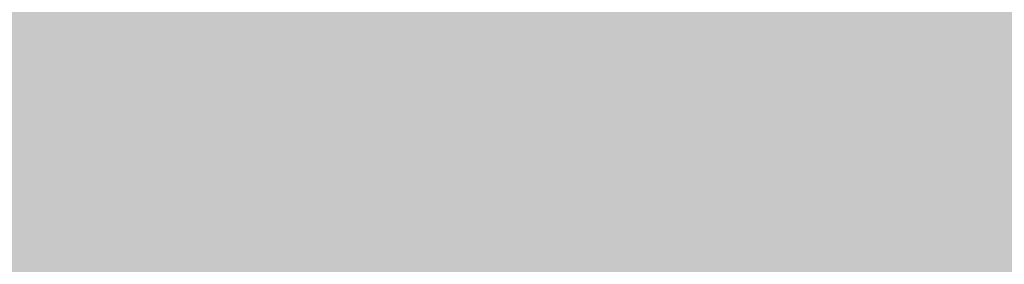
# Model space of a CAD drawing. Units: inches. Extents: x 2083 to 3317, y 1141 to 2115.
# Tile 155 of 256: x 3126.946713 to 3126.955939, y 1263.263648 to 1263.265937. Entities that reach past the tile are written whole.
import ezdxf

# ---------------------------------------------------------------- set-up
doc = ezdxf.new("R2010")
doc.units = ezdxf.units.IN
doc.layers.add('A-ANNO-DIMS', color=2, linetype='Continuous', lineweight=18)
doc.layers.add('A-WALL-PATT', color=251, linetype='Continuous', lineweight=13, true_color=0x636466)
doc.styles.get("Standard").update_dxf_attribs({"font": 'arial.ttf'})
doc.dimstyles.new('ISO-25', dxfattribs={"dimtxt": 12, "dimasz": 12, "dimexe": 1.25, "dimexo": 0.625, "dimtad": 1, "dimlunit": 3, "dimtxsty": 'Standard', "dimcen": 2.5, "dimadec": 0, "dimazin": 0, "dimtfac": 1, "dimtmove": 0, "dimatfit": 3, "dimfxl": 1, "dimarcsym": 0})

# ---------------------------------------------------------------- blocks, each defined once
blk = doc.blocks.new('*D26')
at = {"layer": 'A-ANNO-DIMS', "color": 0, "lineweight": -2, "transparency": 16777216}
for p, q in [((3088.985844, 1274.915092), (3088.985844, 1270.9519631)), ((3111.2400366, 1274.915092), (3111.2400366, 1270.9519631)), ((3076.985844, 1272.2019631), (2840.262447, 1272.2019631)), ((3111.2400366, 1272.2019631), (3088.985844, 1272.2019631)), ((3123.2400366, 1272.2019631), (3135.2400366, 1272.2019631))]:
    blk.add_line(p, q, dxfattribs=at)
at = {"layer": 'A-ANNO-DIMS', "color": 0, "transparency": 16777216}
for points in [[(3076.985844, 1274.2019631), (3076.985844, 1270.2019631), (3088.985844, 1272.2019631)], [(3123.2400366, 1274.2019631), (3123.2400366, 1270.2019631), (3111.2400366, 1272.2019631)]]:
    blk.add_solid(points, dxfattribs=at)
at = {"layer": 'Defpoints', "color": 0, "transparency": 16777216}
for p in [(3088.985844, 1275.540092), (3111.2400366, 1275.540092), (3088.985844, 1272.2019631)]:
    blk.add_point(p, dxfattribs=at)
at = {"layer": 'A-ANNO-DIMS', "color": 0, "transparency": 16777216, "insert": (2952.6241455, 1279.0316016), "char_height": 12, "attachment_point": 5}
blk.add_mtext('NIGHTSTAND 1\'-10 1/2" TYP.', dxfattribs=at)

msp = doc.modelspace()

# ---------------------------------------------------------------- hatches: boundary and pattern name
at = {"layer": 'A-WALL-PATT'}
h = msp.add_hatch(color=256, dxfattribs=at)
h.dxf.hatch_style = 1
h.paths.add_polyline_path([(3126.9597832, 2020.7613601), (2748.9597832, 2020.7613601), (2604.9597832, 2020.7613601), (2226.9597832, 2020.7613601), (2226.9597832, 1702.7613601), (2466.9597832, 1702.7613601), (2466.9597832, 1582.7613601), (2418.9597832, 1582.7613601), (2418.9597832, 1477.7613601), (2226.9597832, 1477.7613601), (2226.9597832, 1263.2613601), (2544.9597832, 1263.2613601), (2544.9597832, 1411.7613601), (2604.9597832, 1411.7613601), (2685.9597832, 1411.7613601), (2685.9597832, 1420.7613601), (2604.9597832, 1420.7613601), (2604.9597832, 1573.7613601), (2604.9597832, 1702.7613601), (2604.9597832, 2011.7613601), (2748.9597832, 2011.7613601), (2748.9597832, 1702.7613601), (2862.9597832, 1702.7613601), (2862.9597832, 1621.7613601), (2871.9597832, 1621.7613601), (2871.9597832, 1702.7613601), (2883.9597832, 1702.7613601), (2883.9597832, 1706.9394595, -0.026459), (2883.9597832, 1711.7613601), (2757.9597832, 1711.7613601), (2757.9597832, 1807.7613601), (2787.9597832, 1807.7613601), (2787.9597832, 1812.2613601), (2757.9597832, 1812.2613601), (2757.9597832, 2011.7613601), (2877.9597832, 2011.7613601), (2877.9597832, 1812.2613601), (2847.9597832, 1812.2613601), (2847.9597832, 1807.7613601), (2889.8357425, 1807.7613601), (2889.8357425, 1812.2613601), (2882.4597832, 1812.2613601), (2882.4597832, 2011.7613601), (3117.9597832, 2011.7613601), (3117.9597832, 1812.2613601), (2937.8357425, 1812.2613601), (2937.8357425, 1807.7613601), (2995.7097832, 1807.7613601), (2995.7097832, 1796.1176655), (3000.2097832, 1796.1176655), (3000.2097832, 1807.7613601), (3117.9597832, 1807.7613601), (3117.9597832, 1711.7613601), (3000.2097832, 1711.7613601), (3000.2097832, 1760.1176655), (2998.5727047, 1760.1176655, -0.020711), (2995.7097832, 1760.1176655), (2995.7097832, 1711.7613601), (2931.9597832, 1711.7613601), (2931.9597832, 1702.7613601), (3126.9597832, 1702.7613601)])
h.paths.add_polyline_path([(2471.4597832, 2011.7613601), (2471.4597832, 1810.0113601), (2462.7169357, 1810.0113601), (2462.7169357, 1805.5113601), (2505.9597832, 1805.5113601), (2505.9597832, 1810.0113601), (2475.9597832, 1810.0113601), (2475.9597832, 2011.7613601), (2595.9597832, 2011.7613601), (2595.9597832, 1810.0113601), (2565.9597832, 1810.0113601), (2565.9597832, 1805.5113601), (2595.9597832, 1805.5113601), (2595.9597832, 1711.7613601), (2235.9597832, 1711.7613601), (2235.9597832, 1805.5113601), (2353.7097832, 1805.5113601), (2353.7097832, 1796.0541624), (2358.2097832, 1796.0541624), (2358.2097832, 1805.5113601), (2414.7169357, 1805.5113601), (2414.7169357, 1810.0113601), (2235.9597832, 1810.0113601), (2235.9597832, 2011.7613601)], flags=16)
h.paths.add_polyline_path([(2270.2047343, 1994.6100082), (2270.2047343, 1970.6100082), (2246.2047343, 1970.6100082), (2246.2047343, 1994.6100082)], flags=0)
edge = h.paths.add_edge_path(flags=0)
edge.add_ellipse((2332.027391, 1899.7981761), major_axis=(-3.0429938, 3.0429938), ratio=0.16825245, start_angle=-161.3321656, end_angle=-156.3071136, ccw=False)
edge.add_ellipse((2333.0820373, 1898.7435297), major_axis=(-1.0546463, 1.0546463), ratio=0.453532097, start_angle=-123.371019, end_angle=-94.1591066)
edge = h.paths.add_edge_path(flags=0)
edge.add_ellipse((2332.027391, 1968.8762897), major_axis=(3.0429938, 3.0429938), ratio=0.16825245, start_angle=18.6678344, end_angle=23.6928864)
edge.add_spline(control_points=[(2332.9255964, 1970.6911045), (2332.2267681, 1970.3360997), (2330.8937087, 1969.6589054), (2328.4130803, 1970.9321376), (2327.2039345, 1967.7487119), (2324.7095965, 1969.9555886), (2322.5328223, 1967.012354), (2320.0128462, 1971.2958124), (2317.6803077, 1968.1578449), (2316.0405263, 1967.1020468), (2315.4269045, 1966.8096022)], knot_values=[0, 0, 0, 0, 2.267059, 4.324559, 6.685584, 8.878641, 11.121502, 14.300359, 17.755284, 19.732645, 19.732645, 19.732645, 19.732645], degree=3, periodic=0)
edge.add_ellipse((2332.027391, 1968.8762897), major_axis=(3.0429938, 3.0429938), ratio=0.16825245, start_angle=18.6678344, end_angle=23.6928864, ccw=False)
edge.add_ellipse((2333.0820373, 1969.930936), major_axis=(1.0546463, 1.0546463), ratio=0.453532097, start_angle=56.628981, end_angle=85.8408934, ccw=False)
edge = h.paths.add_edge_path(flags=0)
edge.add_spline(control_points=[(2296.4282874, 1967.9879081), (2293.6278045, 1965.3363137), (2287.7036238, 1959.727094), (2299.7438601, 1949.9956993), (2294.5325909, 1935.6685275), (2290.5732281, 1920.6035119), (2293.3941244, 1909.9736911), (2296.1854073, 1904.9665431)], knot_values=[0.099185, 0.099185, 0.099185, 0.099185, 0.345301, 0.619822, 0.982653, 1.386093, 1.810555, 1.810555, 1.810555, 1.810555], degree=3, periodic=0)
edge.add_spline(control_points=[(2296.1854073, 1904.9665431), (2297.3835817, 1902.6193002), (2298.0009694, 1901.9493116), (2298.5529698, 1901.4681549)], knot_values=[0.006246, 0.006246, 0.006246, 0.006246, 0.055476, 0.055476, 0.055476, 0.055476], degree=3, periodic=0)
edge.add_spline(control_points=[(2298.5529698, 1901.4681549), (2297.2586121, 1900.9232238), (2295.2252939, 1900.2321257), (2293.0602287, 1900.6142053), (2292.1014227, 1900.788415), (2292.0895776, 1900.790568)], knot_values=[0.312835, 0.312835, 0.312835, 0.312835, 0.40178, 0.474987, 0.475903, 0.475903, 0.475903, 0.475903], degree=3, periodic=0)
edge.add_arc((2292.7936464, 1904.6641088), 3.9370079, 215.4208969, 259.6981795, ccw=False)
edge.add_spline(control_points=[(2289.5853139, 1902.3823039), (2289.4766524, 1902.5350874), (2289.3684805, 1902.6880353), (2289.2608648, 1902.8411699)], knot_values=[0.102872, 0.102872, 0.102872, 0.102872, 0.116896, 0.116896, 0.116896, 0.116896], degree=3, periodic=0)
edge.add_spline(control_points=[(2289.2608648, 1902.8411699), (2288.6866042, 1902.5501922), (2287.6400477, 1902.0199025), (2285.8813368, 1901.8739536), (2283.8529717, 1901.5043521), (2281.7199871, 1899.7105375), (2278.4669913, 1899.492942), (2276.1571361, 1901.8832022), (2272.2589526, 1899.8040711), (2267.7776054, 1901.8431828), (2262.2438819, 1900.1840326), (2257.414927, 1901.7820606), (2254.318374, 1900.7261196), (2253.1782849, 1900.3373431)], knot_values=[0, 0, 0, 0, 1.907977, 3.477176, 5.261074, 7.972851, 11.680248, 13.717921, 16.939592, 22.789562, 27.502503, 33.595215, 37.145618, 37.145618, 37.145618, 37.145618], degree=3, periodic=0)
edge.add_line((2253.1782849, 1900.3373431), (2250.2442397, 1902.8411699))
edge.add_line((2250.2442397, 1902.8411699), (2250.2442397, 1965.8332959))
edge.add_line((2250.2442397, 1965.8332959), (2253.1782849, 1968.3371226))
edge.add_spline(control_points=[(2253.1782849, 1968.3371226), (2254.318374, 1967.9483462), (2257.414927, 1966.8924051), (2262.2438819, 1968.4904332), (2267.7776054, 1966.8312829), (2271.5267301, 1968.5372172), (2273.8759143, 1967.8282895), (2274.2067012, 1967.7276424)], knot_values=[0, 0, 0, 0, 0.09018, 0.244935, 0.364644, 0.513233, 0.537855, 0.537855, 0.537855, 0.537855], degree=3, periodic=0)
edge.add_arc((2274.3528869, 1963.7933495), 3.9370079, 72.0511336, 92.1279492, ccw=False)
edge.add_arc((2281.2969331, 1985.2300027), 18.5962982, 252.05113361, 288.56572166)
edge.add_arc((2292.3167172, 1956.0288805), 12.6460805, 71.02678788, 113.77821843, ccw=False)
edge = h.paths.add_edge_path(flags=0)
edge.add_spline(control_points=[(2274.8994147, 1951.8561946), (2275.066156, 1951.6165924), (2275.2326866, 1951.3765878), (2275.3979871, 1951.1358545)], knot_values=[1.409916, 1.409916, 1.409916, 1.409916, 1.43159, 1.43159, 1.43159, 1.43159], degree=3, periodic=0)
edge.add_spline(control_points=[(2275.3979871, 1951.1358545), (2275.7921055, 1950.5618854), (2276.1792311, 1949.9837745), (2276.5455462, 1949.3971029)], knot_values=[1.358238, 1.358238, 1.358238, 1.358238, 1.409916, 1.409916, 1.409916, 1.409916], degree=3, periodic=0)
edge.add_line((2276.5455462, 1949.3971029), (2277.437289, 1947.8621847))
edge.add_spline(control_points=[(2277.437289, 1947.8621847), (2276.3038341, 1945.6731147), (2274.6396979, 1942.4268817), (2274.631615, 1938.0938998), (2272.7991237, 1930.8515498), (2274.3564261, 1943.8970461), (2275.9476814, 1947.9233558), (2276.5455462, 1949.3971029)], knot_values=[0.005632, 0.005632, 0.005632, 0.005632, 0.186014, 0.266002, 0.357087, 0.59639, 0.739732, 0.739732, 0.739732, 0.739732], degree=3, periodic=0)
edge.add_spline(control_points=[(2276.5455462, 1949.3971029), (2276.1792311, 1949.9837745), (2275.7921055, 1950.5618854), (2275.3979871, 1951.1358545)], knot_values=[1.358238, 1.358238, 1.358238, 1.358238, 1.409916, 1.409916, 1.409916, 1.409916], degree=3, periodic=0)
edge.add_spline(control_points=[(2275.3979871, 1951.1358545), (2274.9425002, 1950.0804523), (2274.2077604, 1948.0252718), (2273.9346018, 1944.8514774), (2272.4685341, 1937.6274891), (2273.4662155, 1945.6964663), (2274.7006154, 1951.0594725), (2274.8994147, 1951.8561946)], knot_values=[0.104364, 0.104364, 0.104364, 0.104364, 0.189636, 0.269624, 0.36071, 0.600013, 0.644622, 0.644622, 0.644622, 0.644622], degree=3, periodic=0)
h.paths.add_polyline_path([(2269.1675139, 1963.1275729, -0.357527), (2268.170633, 1960.9763695, -0.092561), (2268.170633, 1939.4363249, -0.357527), (2269.1675139, 1937.2851215, -0.357527), (2267.0163105, 1938.2820024, -0.164785), (2254.6855813, 1938.2820024, -0.357527), (2252.5343779, 1937.2851215, -0.357527), (2253.5312587, 1939.4363249, -0.092561), (2253.5312587, 1960.9763695, -0.357527), (2252.5343779, 1963.1275729, -0.357527), (2254.6855813, 1962.130692, -0.164785), (2267.0163105, 1962.130692, -0.357527)], flags=0)
h.paths.add_polyline_path([(2248.8740679, 1967.8017998), (2248.8740679, 1957.0277095), (2249.4577833, 1957.0277095), (2249.4577833, 1911.6467562), (2248.8740679, 1911.6467562), (2248.8740679, 1900.8726659), (2246.5118632, 1900.8726659, 0.197327), (2244.1496584, 1902.4568734), (2244.1496584, 1966.2175923, 0.197327), (2246.5118632, 1967.8017998)], flags=0)
h.paths.add_polyline_path([(2269.1675139, 1931.3893442, -0.357527), (2268.170633, 1929.2381408, -0.092561), (2268.170633, 1907.6980962, -0.357527), (2269.1675139, 1905.5468928, -0.357527), (2267.0163105, 1906.5437737, -0.164785), (2254.6855813, 1906.5437737, -0.357527), (2252.5343779, 1905.5468928, -0.357527), (2253.5312587, 1907.6980962, -0.092561), (2253.5312587, 1929.2381408, -0.357527), (2252.5343779, 1931.3893442, -0.357527), (2254.6855813, 1930.3924634, -0.164785), (2267.0163105, 1930.3924634, -0.357527)], flags=0)
edge = h.paths.add_edge_path(flags=0)
edge.add_spline(control_points=[(2276.1968578, 1906.7237016), (2276.1681442, 1909.0289278), (2276.1140492, 1913.371852), (2270.5984171, 1924.9249783), (2273.9051746, 1919.0127787), (2275.9217115, 1916.2620626), (2275.4745699, 1912.4021495), (2277.2578735, 1910.3806206), (2276.6960436, 1908.2250358), (2276.6462176, 1906.8130226), (2276.6178249, 1906.0084068)], knot_values=[0, 0, 0, 0, 8.61026, 16.221274, 18.843057, 23.804898, 27.440828, 29.356102, 31.203478, 33.650687, 33.650687, 33.650687, 33.650687], degree=3, periodic=0)
edge.add_spline(control_points=[(2276.6178249, 1906.0084068), (2276.6233131, 1905.6241436), (2276.4977381, 1904.6286608), (2275.4417789, 1903.8547251), (2274.9373144, 1903.0804497), (2274.8590804, 1902.8411699)], knot_values=[0.156488, 0.156488, 0.156488, 0.156488, 0.184398, 0.231376, 0.250598, 0.250598, 0.250598, 0.250598], degree=3, periodic=0)
edge.add_line((2274.8590804, 1902.8411699), (2276.50598, 1902.8411699))
edge.add_spline(control_points=[(2276.50598, 1902.8411699), (2276.7883084, 1903.0849395), (2277.6650711, 1904.1251958), (2278.2495378, 1904.340738), (2277.6538719, 1908.5273866), (2278.15567, 1906.2278078), (2278.100464, 1905.2859484), (2278.8466748, 1904.0690054), (2277.8567853, 1903.4149482), (2277.8741909, 1902.9910497), (2277.9035616, 1902.8411699)], knot_values=[0.059574, 0.059574, 0.059574, 0.059574, 0.080753, 0.103741, 0.16972, 0.176036, 0.207137, 0.240474, 0.262341, 0.27366, 0.27366, 0.27366, 0.27366], degree=3, periodic=0)
edge.add_line((2277.9035616, 1902.8411699), (2280.0298255, 1902.8411699))
edge.add_spline(control_points=[(2280.0298255, 1902.8411699), (2279.8882214, 1903.088398), (2279.4992571, 1903.9815512), (2280.1522839, 1905.9393491), (2278.103615, 1909.6577572), (2279.7623946, 1907.185285), (2280.3279002, 1904.8748608), (2280.4851086, 1903.4895904), (2281.4632687, 1903.2494323), (2281.7583431, 1902.9364967), (2281.8340361, 1902.8411699)], knot_values=[0.013856, 0.013856, 0.013856, 0.013856, 0.034874, 0.088867, 0.107879, 0.126738, 0.158714, 0.193757, 0.217487, 0.226722, 0.226722, 0.226722, 0.226722], degree=3, periodic=0)
edge.add_spline(control_points=[(2281.8340361, 1902.8411699), (2281.7875348, 1902.8267029), (2281.6470224, 1902.7829881), (2281.3955272, 1902.85949), (2281.088077, 1902.9852418), (2280.7206826, 1903.060902), (2280.3334513, 1903.0257257), (2280.1247668, 1902.898879), (2280.0298255, 1902.8411699)], knot_values=[0, 0, 0, 0, 0.14413, 0.435517, 0.749276, 1.153046, 1.548371, 1.878348, 1.878348, 1.878348, 1.878348], degree=3, periodic=0)
edge.add_line((2280.0298255, 1902.8411699), (2277.9035616, 1902.8411699))
edge.add_spline(control_points=[(2277.9035616, 1902.8411699), (2277.892855, 1902.7958553), (2277.865396, 1902.6796374), (2277.6074793, 1902.6874828), (2277.2740503, 1902.8006999), (2276.8379209, 1902.6197745), (2276.5838074, 1902.7892611), (2276.50598, 1902.8411699)], knot_values=[0, 0, 0, 0, 0.127189, 0.326199, 0.628009, 1.24357, 1.515331, 1.515331, 1.515331, 1.515331], degree=3, periodic=0)
edge.add_line((2276.50598, 1902.8411699), (2274.8590804, 1902.8411699))
edge.add_spline(control_points=[(2274.8590804, 1902.8411699), (2274.8144367, 1902.8985868), (2274.7251297, 1903.013446), (2274.4934765, 1903.1189684), (2274.2442854, 1902.9605386), (2273.9371207, 1903.1849416), (2273.6140395, 1902.9831428), (2273.4083164, 1902.8830449), (2273.322254, 1902.8411699)], knot_values=[0, 0, 0, 0, 0.21843, 0.436957, 0.687977, 0.990379, 1.398396, 1.69185, 1.69185, 1.69185, 1.69185], degree=3, periodic=0)
edge.add_spline(control_points=[(2273.322254, 1902.8411699), (2273.6167403, 1903.445692), (2274.2739977, 1904.5382529), (2276.0272387, 1904.5737017), (2276.2069634, 1906.5836372), (2276.1968578, 1906.7237016)], knot_values=[0.012227, 0.012227, 0.012227, 0.012227, 0.059472, 0.106218, 0.134458, 0.134458, 0.134458, 0.134458], degree=3, periodic=0)
h.paths.add_polyline_path([(2270.7760538, 1897.7898284), (2270.7760538, 1873.7898284), (2246.7760538, 1873.7898284), (2246.7760538, 1897.7898284)], flags=0)
h.paths.add_polyline_path([(2353.7097832, 1760.0050593), (2353.7097832, 1760.0541624), (2358.2097832, 1760.0541624, -0.033729)], flags=0)
h.paths.add_polyline_path([(2321.8191188, 1737.5291862), (2341.9953271, 1737.5291862, -0.414214), (2343.2032727, 1736.3212406), (2343.2032727, 1721.0205964, -0.414214), (2341.9953271, 1719.8126508), (2321.8191188, 1719.8126508, -0.414214), (2320.6111732, 1721.0205964), (2320.6111732, 1736.3212406, -0.414214)], flags=0)
h.paths.add_polyline_path([(2324.2350099, 1736.3212406), (2339.5794359, 1736.3212406, -0.414214), (2341.9953271, 1733.9053494), (2341.9953271, 1725.4497302, -0.414214), (2339.5794359, 1723.033839), (2333.6805885, 1723.033839), (2333.8453172, 1722.0454666, -0.870646), (2335.4253988, 1721.8258934, -0.767327), (2333.922694, 1721.4232449), (2331.2910241, 1721.4232449, -0.767327), (2329.7883193, 1721.8258934, -0.870646), (2331.3684009, 1722.0454666), (2331.5331296, 1723.033839), (2324.2350099, 1723.033839, -0.414214), (2321.8191188, 1725.4497302), (2321.8191188, 1733.9053494, -0.414214)], flags=0)
h.paths.add_polyline_path([(2570.4837892, 1928.6154443), (2589.6837892, 1928.6154443), (2590.1688286, 1928.6154443), (2590.1688286, 1904.9933971), (2570.4837892, 1904.9933971)], flags=0)
h.paths.add_polyline_path([(2574.4473242, 1927.2638215, -1), (2572.8288357, 1927.2638215, -1)], flags=0)
h.paths.add_polyline_path([(2573.0898665, 1926.9408768), (2573.925032, 1927.7760423), (2574.1477428, 1927.5533315), (2573.3125773, 1926.718166)], flags=0)
h.paths.add_polyline_path([(2578.7790648, 1919.7296175, -1), (2571.5916632, 1919.7296175, -1)], flags=0)
h.paths.add_polyline_path([(2578.385364, 1919.7296175, -1), (2571.985364, 1919.7296175, -1)], flags=0)
h.paths.add_polyline_path([(2331.5957638, 1729.4762156, -1), (2333.6179542, 1729.4762156, -1)], flags=0)
h.paths.add_polyline_path([(2578.0342282, 1927.2638215, -1), (2576.4157396, 1927.2638215, -1)], flags=0)
h.paths.add_polyline_path([(2576.6888513, 1927.5310886), (2576.9115621, 1927.7537993), (2577.7467276, 1926.9186339), (2577.5240168, 1926.6959231)], flags=0)
h.paths.add_polyline_path([(2578.1390648, 1909.8595388, -1), (2572.2316632, 1909.8595388, -1)], flags=0)
h.paths.add_polyline_path([(2577.745364, 1909.8595388, -1), (2572.625364, 1909.8595388, -1)], flags=0)
h.paths.add_polyline_path([(2583.7977179, 1927.2638215, -1), (2582.1792294, 1927.2638215, -1)], flags=0)
h.paths.add_polyline_path([(2582.7186487, 1927.7537993), (2583.5538142, 1926.9186339), (2583.3311034, 1926.6959231), (2582.4959379, 1927.5310886)], flags=0)
h.paths.add_polyline_path([(2582.4959379, 1927.5310886), (2582.7186487, 1927.7537993), (2583.5538142, 1926.9186339), (2583.3311034, 1926.6959231)], flags=0)
h.paths.add_polyline_path([(2587.7390648, 1920.5296175, -1), (2581.8316632, 1920.5296175, -1)], flags=0)
h.paths.add_polyline_path([(2587.345364, 1920.5296175, -1), (2582.225364, 1920.5296175, -1)], flags=0)
h.paths.add_polyline_path([(2587.3846219, 1927.2638215, -1), (2585.7661333, 1927.2638215, -1)], flags=0)
h.paths.add_polyline_path([(2586.0819925, 1926.9802469), (2586.917158, 1927.8154124), (2587.1398688, 1927.5927016), (2586.3047033, 1926.7575361)], flags=0)
h.paths.add_polyline_path([(2588.3790648, 1910.6595388, -1), (2581.1916632, 1910.6595388, -1)], flags=0)
h.paths.add_polyline_path([(2587.985364, 1910.6595388, -1), (2581.585364, 1910.6595388, -1)], flags=0)
h.paths.add_polyline_path([(2417.1677288, 1729.4778955), (2437.3439372, 1729.4778955, -0.414214), (2438.5518828, 1728.2699499), (2438.5518828, 1712.9693057, -0.414214), (2437.3439372, 1711.7613601), (2417.1677288, 1711.7613601, -0.414214), (2415.9597832, 1712.9693057), (2415.9597832, 1728.2699499, -0.414214)], flags=0)
h.paths.add_polyline_path([(2419.58362, 1728.2699499), (2434.928046, 1728.2699499, -0.414214), (2437.3439372, 1725.8540587), (2437.3439372, 1717.3984395, -0.414214), (2434.928046, 1714.9825483), (2429.0291985, 1714.9825483), (2429.1939273, 1713.9941758, -0.870646), (2430.7740089, 1713.7746027, -0.767327), (2429.2713041, 1713.3719542), (2426.6396342, 1713.3719542, -0.767327), (2425.1369294, 1713.7746027, -0.870646), (2426.717011, 1713.9941758), (2426.8817397, 1714.9825483), (2419.58362, 1714.9825483, -0.414214), (2417.1677288, 1717.3984395), (2417.1677288, 1725.8540587, -0.414214)], flags=0)
h.paths.add_polyline_path([(2419.58362, 1728.2699499), (2434.928046, 1728.2699499, -0.414214), (2437.3439372, 1725.8540587), (2437.3439372, 1717.3984395, -0.414214), (2434.928046, 1714.9825483), (2429.0291985, 1714.9825483), (2428.3581177, 1719.0090337), (2427.5528206, 1719.0090337), (2426.8817397, 1714.9825483), (2419.58362, 1714.9825483, -0.414214), (2417.1677288, 1717.3984395), (2417.1677288, 1725.8540587, -0.414214)], flags=0)
h.paths.add_polyline_path([(2426.9443739, 1721.4249248, -1), (2428.9665643, 1721.4249248, -1)], flags=0)
h.paths.add_polyline_path([(2475.9597832, 1702.7613601), (2595.9597832, 1702.7613601), (2595.9597832, 1582.7613601), (2475.9597832, 1582.7613601)], flags=16)
h.paths.add_polyline_path([(2427.9597832, 1573.7613601), (2595.9597832, 1573.7613601), (2595.9597832, 1468.7613601), (2595.9597832, 1420.7613601), (2384.4597832, 1420.7613601), (2384.4597832, 1468.7613601), (2427.9597832, 1468.7613601)], flags=16)
h.paths.add_polyline_path([(2379.9597832, 1468.7613601), (2379.9597832, 1420.7613601), (2235.9597832, 1420.7613601), (2235.9597832, 1468.7613601)], flags=16)
h.paths.add_polyline_path([(2317.8159962, 1466.695767), (2337.9922045, 1466.695767, -0.414214), (2339.2001501, 1465.4878214), (2339.2001501, 1450.1871771, -0.414214), (2337.9922045, 1448.9792315), (2317.8159962, 1448.9792315, -0.414214), (2316.6080506, 1450.1871771), (2316.6080506, 1465.4878214, -0.414214)], flags=0)
h.paths.add_polyline_path([(2320.2318874, 1465.4878214), (2335.5763133, 1465.4878214, -0.414214), (2337.9922045, 1463.0719302), (2337.9922045, 1454.616311, -0.414214), (2335.5763133, 1452.2004198), (2329.6774659, 1452.2004198), (2329.8421946, 1451.2120473, -0.870646), (2331.4222762, 1450.9924742, -0.767327), (2329.9195714, 1450.5898257), (2327.2879015, 1450.5898257, -0.767327), (2325.7851967, 1450.9924742, -0.870646), (2327.3652783, 1451.2120473), (2327.530007, 1452.2004198), (2320.2318874, 1452.2004198, -0.414214), (2317.8159962, 1454.616311), (2317.8159962, 1463.0719302, -0.414214)], flags=0)
h.paths.add_polyline_path([(2320.2318874, 1465.4878214), (2335.5763133, 1465.4878214, -0.414214), (2337.9922045, 1463.0719302), (2337.9922045, 1454.616311, -0.414214), (2335.5763133, 1452.2004198), (2329.6774659, 1452.2004198), (2329.006385, 1456.2269051), (2328.2010879, 1456.2269051), (2327.530007, 1452.2004198), (2320.2318874, 1452.2004198, -0.414214), (2317.8159962, 1454.616311), (2317.8159962, 1463.0719302, -0.414214)], flags=0)
h.paths.add_polyline_path([(2327.5926413, 1458.6427963, -1), (2329.6148317, 1458.6427963, -1)], flags=0)
h.paths.add_polyline_path([(2244.4117436, 1433.3404531), (2241.9209449, 1433.3404531, -0.414214), (2240.0178562, 1435.2435418), (2240.0178562, 1440.9528078, -0.414211), (2241.920925, 1442.8558965), (2244.4117436, 1442.8558965, -1.976472)], flags=0)
h.paths.add_polyline_path([(2245.3568884, 1434.3975358, -0.414214), (2245.3568884, 1441.7988138, -2.144098)], flags=0)
h.paths.add_polyline_path([(2535.9597832, 1416.2613601), (2535.9597832, 1272.2613601), (2235.9597832, 1272.2613601), (2235.9597832, 1416.2613601)], flags=16)
h.paths.add_polyline_path([(2260.1195614, 1384.2928413), (2260.1195614, 1362.0386487), (2237.8653688, 1362.0386487), (2237.8653688, 1384.2928413)], flags=0)
edge = h.paths.add_edge_path(flags=0)
edge.add_line((2318.2518466, 1362.0932983), (2318.1457968, 1362.0009726))
edge.add_ellipse((2317.4451158, 1360.4310442), major_axis=(2.8216404, 2.8216404), ratio=0.16825245, start_angle=18.6678344, end_angle=20.9481273, ccw=False)
edge.add_ellipse((2318.4230451, 1361.4089735), major_axis=(0.9779293, 0.9779293), ratio=0.453532097, start_angle=56.628981, end_angle=70.2262012, ccw=False)
edge = h.paths.add_edge_path(flags=0)
edge.add_line((2319.1073699, 1295.5710784), (2319.0150442, 1295.6771282))
edge.add_ellipse((2317.4451158, 1296.3778091), major_axis=(-2.8216404, 2.8216404), ratio=0.16825245, start_angle=-161.3321656, end_angle=-159.0518727, ccw=False)
edge.add_ellipse((2318.4230451, 1295.3998798), major_axis=(-0.9779293, 0.9779293), ratio=0.453532097, start_angle=-123.371019, end_angle=-109.7737988)
edge = h.paths.add_edge_path(flags=0)
edge.add_spline(control_points=[(2284.2103489, 1301.1702189), (2284.5806878, 1300.444719), (2284.8911891, 1299.8920243), (2285.159553, 1299.4610182)], knot_values=[0.039066, 0.039066, 0.039066, 0.039066, 0.055476, 0.055476, 0.055476, 0.055476], degree=3, periodic=0)
edge.add_line((2285.159553, 1299.4610182), (2284.2103489, 1301.1702189))
edge = h.paths.add_edge_path(flags=0)
edge.add_line((2280.4124579, 1297.2980125), (2283.3699905, 1297.0361216))
edge.add_line((2283.3699905, 1297.0361216), (2286.4056902, 1297.9263104))
edge.add_spline(control_points=[(2286.4056902, 1297.9263104), (2285.305487, 1297.4631193), (2284.3447774, 1297.1291508), (2283.3699905, 1297.0361216)], knot_values=[0.394369, 0.394369, 0.394369, 0.394369, 0.475903, 0.475903, 0.475903, 0.475903], degree=3, periodic=0)
edge.add_spline(control_points=[(2283.3699905, 1297.0361216), (2283.2813895, 1297.027666), (2282.316289, 1296.9573356), (2281.3125019, 1297.1344787), (2280.4234414, 1297.2960161), (2280.4124579, 1297.2980125)], knot_values=[0.312835, 0.312835, 0.312835, 0.312835, 0.320246, 0.393453, 0.394369, 0.394369, 0.394369, 0.394369], degree=3, periodic=0)
edge = h.paths.add_edge_path(flags=0)
edge.add_line((2284.4355615, 1359.6072854), (2280.4462909, 1355.328047))
edge.add_line((2280.4462909, 1355.328047), (2279.5799868, 1351.0177544))
edge.add_line((2279.5799868, 1351.0177544), (2282.4129737, 1346.5804327))
edge.add_spline(control_points=[(2282.4129737, 1346.5804327), (2283.1533308, 1345.5892358), (2284.2528957, 1344.0288973), (2284.801037, 1342.3871671), (2284.9351625, 1341.8055443)], knot_values=[1.240098, 1.240098, 1.240098, 1.240098, 1.332892, 1.382712, 1.382712, 1.382712, 1.382712], degree=3, periodic=0)
edge.add_spline(control_points=[(2284.9351625, 1341.8055443), (2285.3191079, 1340.1406002), (2285.2330291, 1338.4092041), (2284.9099384, 1336.6541222)], knot_values=[1.097484, 1.097484, 1.097484, 1.097484, 1.240098, 1.240098, 1.240098, 1.240098], degree=3, periodic=0)
edge.add_spline(control_points=[(2284.9099384, 1336.6541222), (2284.5868478, 1334.8990403), (2284.0267453, 1333.1202725), (2283.4626437, 1331.3605849)], knot_values=[0.95487, 0.95487, 0.95487, 0.95487, 1.097484, 1.097484, 1.097484, 1.097484], degree=3, periodic=0)
edge.add_line((2283.4626437, 1331.3605849), (2281.8903759, 1326.153357))
edge.add_line((2281.8903759, 1326.153357), (2280.7562592, 1321.0560888))
edge.add_line((2280.7562592, 1321.0560888), (2280.2992048, 1316.0019772))
edge.add_line((2280.2992048, 1316.0019772), (2280.7159327, 1310.9500678))
edge.add_line((2280.7159327, 1310.9500678), (2282.0280939, 1305.9721367))
edge.add_line((2282.0280939, 1305.9721367), (2284.2103489, 1301.1702189))
edge.add_spline(control_points=[(2284.2103489, 1301.1702189), (2283.3407305, 1302.7301854), (2282.6119044, 1304.3364933), (2282.0280939, 1305.9721367)], knot_values=[0.099185, 0.099185, 0.099185, 0.099185, 0.241799, 0.241799, 0.241799, 0.241799], degree=3, periodic=0)
edge.add_spline(control_points=[(2282.0280939, 1305.9721367), (2281.4442835, 1307.6077801), (2281.0054886, 1309.2727591), (2280.7159327, 1310.9500678)], knot_values=[0.241799, 0.241799, 0.241799, 0.241799, 0.384413, 0.384413, 0.384413, 0.384413], degree=3, periodic=0)
edge.add_spline(control_points=[(2280.7159327, 1310.9500678), (2280.4332411, 1312.5876134), (2280.2893863, 1314.2769594), (2280.2988938, 1315.9620324), (2280.2992048, 1316.0019772)], knot_values=[0.384413, 0.384413, 0.384413, 0.384413, 0.523647, 0.527028, 0.527028, 0.527028, 0.527028], degree=3, periodic=0)
edge.add_spline(control_points=[(2280.2992048, 1316.0019772), (2280.3123257, 1317.6869552), (2280.4778706, 1319.3679256), (2280.7562592, 1321.0560888)], knot_values=[0.527028, 0.527028, 0.527028, 0.527028, 0.669642, 0.669642, 0.669642, 0.669642], degree=3, periodic=0)
edge.add_spline(control_points=[(2280.7562592, 1321.0560888), (2281.0346478, 1322.7442519), (2281.4258801, 1324.4396079), (2281.8903759, 1326.153357)], knot_values=[0.669642, 0.669642, 0.669642, 0.669642, 0.812256, 0.812256, 0.812256, 0.812256], degree=3, periodic=0)
edge.add_spline(control_points=[(2281.8903759, 1326.153357), (2282.2643834, 1327.5332507), (2282.7878702, 1329.2618097), (2283.352751, 1331.0177803), (2283.4626437, 1331.3605849)], knot_values=[0.812256, 0.812256, 0.812256, 0.812256, 0.927087, 0.95487, 0.95487, 0.95487, 0.95487], degree=3, periodic=0)
edge.add_line((2283.4626437, 1331.3605849), (2284.9099384, 1336.6541222))
edge.add_line((2284.9099384, 1336.6541222), (2284.9351625, 1341.8055443))
edge.add_line((2284.9351625, 1341.8055443), (2282.4129737, 1346.5804327))
edge.add_spline(control_points=[(2282.4129737, 1346.5804327), (2281.2751273, 1348.1037918), (2280.0784467, 1349.5703178), (2279.5799868, 1351.0177544)], knot_values=[1.382712, 1.382712, 1.382712, 1.382712, 1.525326, 1.525326, 1.525326, 1.525326], degree=3, periodic=0)
edge.add_spline(control_points=[(2279.5799868, 1351.0177544), (2279.4432818, 1351.4147209), (2279.1363124, 1352.856922), (2279.7351897, 1354.2903851), (2280.4462909, 1355.328047)], knot_values=[1.525326, 1.525326, 1.525326, 1.525326, 1.564439, 1.667941, 1.667941, 1.667941, 1.667941], degree=3, periodic=0)
edge.add_spline(control_points=[(2280.4462909, 1355.328047), (2281.4261132, 1356.7578354), (2282.9308373, 1358.1825604), (2284.4355615, 1359.6072854)], knot_values=[1.667941, 1.667941, 1.667941, 1.667941, 1.810555, 1.810555, 1.810555, 1.810555], degree=3, periodic=0)
edge.add_arc((2280.6230749, 1348.518181), 11.7261796, 71.02678788, 113.77821843)
edge.add_arc((2270.4048917, 1375.5951559), 17.2435667, 252.05113361, 288.56572166, ccw=False)
edge.add_arc((2263.9659692, 1355.7178471), 3.6506221, 72.0511336, 92.1279492)
edge.add_arc((2263.9659692, 1355.7178471), 3.6506221, 92.1279492, 177.98513)
edge.add_spline(control_points=[(2260.3176041, 1355.8461989), (2260.2604169, 1354.2206683), (2260.551278, 1350.1865469), (2262.9993445, 1346.7662507), (2264.4727415, 1344.6490245)], knot_values=[1.43159, 1.43159, 1.43159, 1.43159, 1.564144, 1.770695, 1.770695, 1.770695, 1.770695], degree=3, periodic=0)
edge.add_line((2264.4727415, 1344.6490245), (2264.9355904, 1343.9825301))
edge.add_spline(control_points=[(2263.8010444, 1340.2481052), (2263.8432379, 1340.5140884), (2264.0672444, 1341.7564652), (2264.5126928, 1343.0024532), (2264.9350468, 1343.9810834)], knot_values=[0.53657, 0.53657, 0.53657, 0.53657, 0.559349, 0.644622, 0.644622, 0.644622, 0.644622], degree=3, periodic=0)
edge.add_spline(control_points=[(2264.9350468, 1343.9810834), (2265.1177715, 1343.7149747), (2265.2988751, 1343.4479058), (2265.4767562, 1343.1793646)], knot_values=[1.384077, 1.384077, 1.384077, 1.384077, 1.409916, 1.409916, 1.409916, 1.409916], degree=3, periodic=0)
edge.add_spline(control_points=[(2265.4767562, 1343.1793646), (2265.6546373, 1342.9108234), (2265.8292958, 1342.64081), (2265.9991301, 1342.368812)], knot_values=[1.358238, 1.358238, 1.358238, 1.358238, 1.384077, 1.384077, 1.384077, 1.384077], degree=3, periodic=0)
edge.add_line((2265.9991301, 1342.368812), (2266.8260057, 1340.9455468))
edge.add_spline(control_points=[(2266.8260057, 1340.9455468), (2268.894401, 1337.0896912), (2271.3981727, 1325.8430009), (2270.5161644, 1310.5685568), (2275.9193759, 1301.860609), (2277.7895113, 1299.1994495)], knot_values=[0.116896, 0.116896, 0.116896, 0.116896, 0.472987, 1.050969, 1.313793, 1.313793, 1.313793, 1.313793], degree=3, periodic=0)
edge.add_spline(control_points=[(2277.7895113, 1299.1994495), (2277.8394051, 1299.1284519), (2277.8894277, 1299.0574975), (2277.9395717, 1298.9865839)], knot_values=[0.109884, 0.109884, 0.109884, 0.109884, 0.116896, 0.116896, 0.116896, 0.116896], degree=3, periodic=0)
edge.add_line((2277.9395717, 1298.9865839), (2277.7888489, 1299.1991139))
edge.add_spline(control_points=[(2277.7888489, 1299.1991139), (2277.2565819, 1298.9294144), (2276.2863504, 1298.4379024), (2275.0393517, 1298.3344186), (2274.3833299, 1298.2388951), (2274.2152543, 1298.209338)], knot_values=[33.12187, 33.12187, 33.12187, 33.12187, 35.029056, 36.598255, 37.144827, 37.144827, 37.144827, 37.144827], degree=3, periodic=0)
edge.add_line((2274.2152543, 1298.209338), (2273.073147, 1297.8929607))
edge.add_spline(control_points=[(2273.073147, 1297.8929607), (2272.3229363, 1297.579784), (2271.0391507, 1296.5105078), (2269.2483948, 1296.2260622), (2268.4231004, 1296.3746543)], knot_values=[26.532584, 26.532584, 26.532584, 26.532584, 29.198919, 31.839101, 31.839101, 31.839101, 31.839101], degree=3, periodic=0)
edge.add_line((2268.4231004, 1296.3746543), (2263.8785014, 1297.4575338))
edge.add_spline(control_points=[(2263.8785014, 1297.4575338), (2263.5560769, 1297.3594345), (2261.8603064, 1296.8386943), (2260.2387805, 1297.2824073), (2258.9334543, 1297.5164611)], knot_values=[15.919551, 15.919551, 15.919551, 15.919551, 16.939592, 21.226067, 21.226067, 21.226067, 21.226067], degree=3, periodic=0)
edge.add_line((2258.9334543, 1297.5164611), (2254.0552332, 1297.3290098))
edge.add_spline(control_points=[(2254.0552332, 1297.3290098), (2253.7555255, 1297.295815), (2252.1136834, 1297.1651738), (2250.4618687, 1297.5442209), (2249.1296862, 1297.6678818)], knot_values=[5.306517, 5.306517, 5.306517, 5.306517, 6.276435, 10.613034, 10.613034, 10.613034, 10.613034], degree=3, periodic=0)
edge.add_line((2249.1296862, 1297.6678818), (2244.3316495, 1296.8777561))
edge.add_line((2244.3316495, 1296.8777561), (2241.6110326, 1299.1994495))
edge.add_line((2241.6110326, 1299.1994495), (2241.6110326, 1357.6094038))
edge.add_line((2241.6110326, 1357.6094038), (2244.3316495, 1359.9310973))
edge.add_line((2244.3316495, 1359.9310973), (2252.7288228, 1359.5426917))
edge.add_spline(control_points=[(2252.7288228, 1359.5426917), (2252.8709387, 1359.5464396), (2253.3057402, 1359.5481716), (2253.7398447, 1359.5142744), (2254.0317419, 1359.4824261)], knot_values=[0.233291, 0.233291, 0.233291, 0.233291, 0.244935, 0.268927, 0.268927, 0.268927, 0.268927], degree=3, periodic=0)
edge.add_line((2254.0317419, 1359.4824261), (2259.5871899, 1359.4163899))
edge.add_spline(control_points=[(2259.5871899, 1359.4163899), (2260.6770676, 1359.6285026), (2262.0731971, 1359.8970025), (2263.5236925, 1359.4592776), (2263.8304173, 1359.3659518)], knot_values=[0.422516, 0.422516, 0.422516, 0.422516, 0.513233, 0.537855, 0.537855, 0.537855, 0.537855], degree=3, periodic=0)
edge.add_arc((2263.9659692, 1355.7178471), 3.6506221, 72.0511336, 92.1279492, ccw=False)
edge.add_arc((2270.4048917, 1375.5951559), 17.2435667, 252.05113361, 288.56572166)
edge.add_arc((2280.6230749, 1348.518181), 11.7261796, 71.02678788, 113.77821843, ccw=False)
h.paths.add_polyline_path([(2240.3405298, 1359.4347149), (2240.3405298, 1349.4443532), (2240.8817846, 1349.4443532), (2240.8817846, 1307.3645001), (2240.3405298, 1307.3645001), (2240.3405298, 1297.3741385), (2238.1501565, 1297.3741385, 0.197327), (2235.9597832, 1298.8431076), (2235.9597832, 1357.9657458, 0.197327), (2238.1501565, 1359.4347149)], flags=0)
h.paths.add_polyline_path([(2259.1577904, 1355.1005005, -0.357527), (2258.2334246, 1353.1057799, -0.092561), (2258.2334246, 1333.1326007, -0.357527), (2259.1577904, 1331.1378801, -0.357527), (2257.1630698, 1332.0622458, -0.164785), (2245.7293022, 1332.0622458, -0.357527), (2243.7345816, 1331.1378801, -0.357527), (2244.6589474, 1333.1326007, -0.092561), (2244.6589474, 1353.1057799, -0.357527), (2243.7345816, 1355.1005005, -0.357527), (2245.7293022, 1354.1761347, -0.164785), (2257.1630698, 1354.1761347, -0.357527)], flags=0)
edge = h.paths.add_edge_path(flags=0)
edge.add_line((2265.9991301, 1342.368812), (2266.8260057, 1340.9455468))
edge.add_line((2266.8260057, 1340.9455468), (2265.3075567, 1337.8140664))
edge.add_line((2265.3075567, 1337.8140664), (2264.358232, 1334.6529388))
edge.add_line((2264.358232, 1334.6529388), (2264.2620123, 1333.7997046))
edge.add_spline(control_points=[(2264.2620123, 1333.7997046), (2264.2083565, 1333.187055), (2264.1620602, 1332.3655252), (2264.0071444, 1331.4139326), (2263.9690487, 1331.2018338)], knot_values=[0.464444, 0.464444, 0.464444, 0.464444, 0.516691, 0.531608, 0.531608, 0.531608, 0.531608], degree=3, periodic=0)
edge.add_spline(control_points=[(2263.9690487, 1331.2018338), (2263.7745349, 1330.1188727), (2263.4243703, 1328.7908386), (2263.2574202, 1328.5306516), (2263.2340282, 1328.5146115)], knot_values=[0.372682, 0.372682, 0.372682, 0.372682, 0.44885, 0.464444, 0.464444, 0.464444, 0.464444], degree=3, periodic=0)
edge.add_spline(control_points=[(2263.2340282, 1328.5146115), (2263.096382, 1328.4202271), (2263.1311696, 1329.3014765), (2263.2749528, 1330.6157493)], knot_values=[0.280919, 0.280919, 0.280919, 0.280919, 0.372682, 0.372682, 0.372682, 0.372682], degree=3, periodic=0)
edge.add_spline(control_points=[(2263.2749528, 1330.6157493), (2263.4187361, 1331.930022), (2263.6715151, 1333.677318), (2263.9698519, 1335.3150268)], knot_values=[0.189157, 0.189157, 0.189157, 0.189157, 0.280919, 0.280919, 0.280919, 0.280919], degree=3, periodic=0)
edge.add_spline(control_points=[(2263.9698519, 1335.3150268), (2264.1004958, 1336.0321917), (2264.4187827, 1337.6219113), (2264.7548476, 1338.8644304), (2264.9474193, 1339.4911244)], knot_values=[0.097394, 0.097394, 0.097394, 0.097394, 0.137578, 0.189157, 0.189157, 0.189157, 0.189157], degree=3, periodic=0)
edge.add_spline(control_points=[(2264.9474193, 1339.4911244), (2265.2900171, 1340.6060546), (2265.6442376, 1341.4939958), (2265.9991301, 1342.368812)], knot_values=[0.005632, 0.005632, 0.005632, 0.005632, 0.097394, 0.097394, 0.097394, 0.097394], degree=3, periodic=0)
h.paths.add_polyline_path([(2259.1577904, 1325.6709733, -0.357527), (2258.2334246, 1323.6762527, -0.092561), (2258.2334246, 1303.7030735, -0.357527), (2259.1577904, 1301.7083529, -0.357527), (2257.1630698, 1302.6327186, -0.164785), (2245.7293022, 1302.6327186, -0.357527), (2243.7345816, 1301.7083529, -0.357527), (2244.6589474, 1303.7030735, -0.092561), (2244.6589474, 1323.6762527, -0.357527), (2243.7345816, 1325.6709733, -0.357527), (2245.7293022, 1324.7466075, -0.164785), (2257.1630698, 1324.7466075, -0.357527)], flags=0)
edge = h.paths.add_edge_path(flags=0)
edge.add_spline(control_points=[(2261.7089377, 1317.3114208), (2261.6794818, 1317.4175798), (2261.7618581, 1317.3885347), (2262.4907358, 1316.0898725), (2262.962185, 1315.3008975)], knot_values=[14.955861, 14.955861, 14.955861, 14.955861, 16.221274, 18.694826, 18.694826, 18.694826, 18.694826], degree=3, periodic=0)
edge.add_spline(control_points=[(2262.962185, 1315.3008975), (2262.9904374, 1315.2536169), (2263.7020958, 1314.0673762), (2264.3489834, 1313.1271533), (2264.7300545, 1312.1641544)], knot_values=[18.694826, 18.694826, 18.694826, 18.694826, 18.843057, 22.433791, 22.433791, 22.433791, 22.433791], degree=3, periodic=0)
edge.add_spline(control_points=[(2264.7300545, 1312.1641544), (2264.8755649, 1311.7964373), (2265.1768733, 1310.7698073), (2265.1430689, 1309.5592623), (2265.2477363, 1308.8241926)], knot_values=[22.433791, 22.433791, 22.433791, 22.433791, 23.804898, 26.172756, 26.172756, 26.172756, 26.172756], degree=3, periodic=0)
edge.add_line((2265.2477363, 1308.8241926), (2265.8507741, 1307.1718879))
edge.add_spline(control_points=[(2265.8507741, 1307.1718879), (2266.0650246, 1306.8216779), (2266.3843872, 1306.3322461), (2266.4244001, 1305.7805489), (2266.4203688, 1305.6112163)], knot_values=[28.062562, 28.062562, 28.062562, 28.062562, 29.356102, 29.911721, 29.911721, 29.911721, 29.911721], degree=3, periodic=0)
edge.add_spline(control_points=[(2266.4203688, 1305.6112163), (2266.4161162, 1305.4325896), (2266.393999, 1305.2499979), (2266.3647773, 1305.0658571)], knot_values=[29.911721, 29.911721, 29.911721, 29.911721, 30.497837, 30.497837, 30.497837, 30.497837], degree=3, periodic=0)
edge.add_line((2266.3647773, 1305.0658571), (2266.0661511, 1302.1362954))
edge.add_spline(control_points=[(2266.0661511, 1302.1362954), (2266.0712401, 1301.7799843), (2265.9980761, 1301.1999847), (2265.6632664, 1300.7589613), (2265.5089084, 1300.5858824)], knot_values=[0.156488, 0.156488, 0.156488, 0.156488, 0.184398, 0.203543, 0.203543, 0.203543, 0.203543], degree=3, periodic=0)
edge.add_line((2265.5089084, 1300.5858824), (2264.4353411, 1299.1994495))
edge.add_line((2264.4353411, 1299.1994495), (2265.962442, 1299.1994495))
edge.add_line((2265.962442, 1299.1994495), (2267.3359898, 1301.1752758))
edge.add_line((2267.3359898, 1301.1752758), (2267.3116668, 1301.9862366))
edge.add_spline(control_points=[(2267.3116668, 1301.9862366), (2267.261111, 1302.8623959), (2267.1602121, 1303.7371316), (2267.2714865, 1303.3258962)], knot_values=[0.126229, 0.126229, 0.126229, 0.126229, 0.166617, 0.166617, 0.166617, 0.166617], degree=3, periodic=0)
edge.add_spline(control_points=[(2267.2714865, 1303.3258962), (2267.2800347, 1303.2943047), (2267.3097851, 1303.1753659), (2267.3734504, 1302.8836084), (2267.4061233, 1302.6828291), (2267.4179259, 1302.6010251)], knot_values=[0.166617, 0.166617, 0.166617, 0.166617, 0.16972, 0.176036, 0.180765, 0.180765, 0.180765, 0.180765], degree=3, periodic=0)
edge.add_spline(control_points=[(2267.7438914, 1300.9875045), (2267.6875832, 1301.1509426), (2267.4805198, 1301.6566644), (2267.4837514, 1302.1447877), (2267.4179259, 1302.6010251)], knot_values=[0.180765, 0.180765, 0.180765, 0.180765, 0.193767, 0.220139, 0.220139, 0.220139, 0.220139], degree=3, periodic=0)
edge.add_line((2267.4179259, 1302.6010251), (2267.7438914, 1300.9875045))
edge.add_spline(control_points=[(2267.7438914, 1300.9875045), (2267.8319608, 1300.7318778), (2267.9320205, 1300.3099042), (2267.5548409, 1299.9745185), (2267.429366, 1299.8292073)], knot_values=[0.220139, 0.220139, 0.220139, 0.220139, 0.240474, 0.25489, 0.25489, 0.25489, 0.25489], degree=3, periodic=0)
edge.add_line((2267.429366, 1299.8292073), (2267.2583608, 1299.1994495))
edge.add_line((2267.2583608, 1299.1994495), (2269.229956, 1299.1994495))
edge.add_spline(control_points=[(2269.229956, 1299.1994495), (2269.0986525, 1299.4286938), (2268.842774, 1300.0162509), (2269.0115749, 1300.9159235), (2268.9467957, 1301.6607397)], knot_values=[0.013856, 0.013856, 0.013856, 0.013856, 0.034874, 0.067073, 0.067073, 0.067073, 0.067073], degree=3, periodic=0)
edge.add_line((2268.9467957, 1301.6607397), (2268.4315815, 1303.6031089))
edge.add_spline(control_points=[(2268.4315815, 1303.6031089), (2268.1755957, 1304.1923747), (2267.5962136, 1305.2512977), (2268.0406981, 1304.6232098), (2268.2513938, 1304.2824205)], knot_values=[0.090155, 0.090155, 0.090155, 0.090155, 0.107879, 0.120289, 0.120289, 0.120289, 0.120289], degree=3, periodic=0)
edge.add_spline(control_points=[(2268.2513938, 1304.2824205), (2268.3608818, 1304.1053294), (2269.0577527, 1302.9179833), (2269.382691, 1301.5904186), (2269.5214051, 1300.7759312), (2269.5752202, 1300.5557836)], knot_values=[0.120289, 0.120289, 0.120289, 0.120289, 0.126738, 0.158714, 0.173506, 0.173506, 0.173506, 0.173506], degree=3, periodic=0)
edge.add_line((2269.5752202, 1300.5557836), (2270.6857984, 1299.4212579))
edge.add_spline(control_points=[(2270.6857984, 1299.4212579), (2270.7672206, 1299.3572512), (2270.8378523, 1299.2814011), (2270.9029248, 1299.1994495)], knot_values=[0.21816, 0.21816, 0.21816, 0.21816, 0.226722, 0.226722, 0.226722, 0.226722], degree=3, periodic=0)
edge.add_line((2270.9372012, 1299.1929131), (2270.9029248, 1299.1994495))
edge.add_spline(control_points=[(2270.9029248, 1299.1994495), (2270.8598061, 1299.1860349), (2270.7295148, 1299.1455), (2270.4963139, 1299.216437), (2270.2716612, 1299.3083234), (2270.1210168, 1299.3479612), (2270.0633386, 1299.3595566)], knot_values=[0.939174, 0.939174, 0.939174, 0.939174, 1.083304, 1.374691, 1.68845, 1.878348, 1.878348, 1.878348, 1.878348], degree=3, periodic=0)
edge.add_line((2270.0633386, 1299.3595566), (2269.229956, 1299.1994495))
edge.add_line((2269.229956, 1299.1994495), (2267.2583608, 1299.1994495))
edge.add_spline(control_points=[(2267.2583608, 1299.1994495), (2267.248433, 1299.1574312), (2267.2229714, 1299.0496673), (2266.9838161, 1299.056942), (2266.8092097, 1299.1162303), (2266.6769047, 1299.1090913), (2266.636531, 1299.1048147)], knot_values=[0.757665, 0.757665, 0.757665, 0.757665, 0.884854, 1.083864, 1.385675, 1.515331, 1.515331, 1.515331, 1.515331], degree=3, periodic=0)
edge.add_spline(control_points=[(2266.636531, 1299.1048147), (2266.4852248, 1299.0887878), (2266.2358066, 1299.0171229), (2266.0346081, 1299.1513168), (2265.962442, 1299.1994495)], knot_values=[0, 0, 0, 0, 0.485905, 0.757665, 0.757665, 0.757665, 0.757665], degree=3, periodic=0)
edge.add_line((2265.962442, 1299.1994495), (2264.4353411, 1299.1994495))
edge.add_line((2264.4353411, 1299.1994495), (2263.8584442, 1299.3671176))
edge.add_spline(control_points=[(2263.8584442, 1299.3671176), (2263.8189433, 1299.3709053), (2263.7795277, 1299.3857212), (2263.7401308, 1299.4015039)], knot_values=[0.845925, 0.845925, 0.845925, 0.845925, 0.978627, 0.978627, 0.978627, 0.978627], degree=3, periodic=0)
edge.add_line((2263.7217862, 1299.3964251), (2263.0103065, 1299.1994495))
edge.add_spline(control_points=[(2263.0103065, 1299.1994495), (2263.2457942, 1299.682859), (2263.5060317, 1300.1281072), (2263.8734943, 1300.4080279)], knot_values=[0.012227, 0.012227, 0.012227, 0.012227, 0.052971, 0.052971, 0.052971, 0.052971], degree=3, periodic=0)
edge.add_spline(control_points=[(2263.8734943, 1300.4080279), (2263.932131, 1300.4526954), (2264.0842429, 1300.5529789), (2264.2551889, 1300.6242227), (2264.3596855, 1300.6647475)], knot_values=[0.052971, 0.052971, 0.052971, 0.052971, 0.059472, 0.069086, 0.069086, 0.069086, 0.069086], degree=3, periodic=0)
edge.add_line((2264.3596855, 1300.6647475), (2265.1418998, 1301.0777737))
edge.add_line((2265.1418998, 1301.0777737), (2265.675806, 1302.7995583))
edge.add_line((2265.675806, 1302.7995583), (2265.5407004, 1305.7040662))
edge.add_line((2265.5407004, 1305.7040662), (2264.8030733, 1309.3277237))
edge.add_line((2264.8030733, 1309.3277237), (2263.0405349, 1314.0917906))
edge.add_spline(control_points=[(2263.0405349, 1314.0917906), (2262.3835724, 1315.6714379), (2261.7959724, 1316.9977489), (2261.7089377, 1317.3114208)], knot_values=[11.216896, 11.216896, 11.216896, 11.216896, 14.955861, 14.955861, 14.955861, 14.955861], degree=3, periodic=0)
h.paths.add_polyline_path([(2871.9597832, 1416.2613601), (2895.910047, 1416.2613601), (2895.910047, 1420.7613601), (2871.9597832, 1420.7613601), (2871.9597832, 1501.7613601), (2862.9597832, 1501.7613601), (2862.9597832, 1420.7613601), (2805.9597832, 1420.7613601), (2805.9597832, 1411.7613601), (2862.9597832, 1411.7613601), (2862.9597832, 1263.2613601), (3126.9597832, 1263.2613601), (3126.9597832, 1411.7613601), (3126.9597832, 1486.7613601), (2943.9597832, 1486.7613601), (2943.9597832, 1477.7613601), (2967.8603109, 1477.7613601), (2967.8603109, 1420.7613601), (2943.910047, 1420.7613601), (2943.910047, 1416.2613601), (3117.9597832, 1416.2613601), (3117.9597832, 1420.7613601), (2972.3603109, 1420.7613601), (2972.3603109, 1477.7613601), (3117.9597832, 1477.7613601), (3117.9597832, 1420.7613601), (3117.9597832, 1272.2613601), (2871.9597832, 1272.2613601)], flags=0)
h.paths.add_polyline_path([(2457.1256256, 1485.9425054), (2527.6026508, 1485.9425054), (2527.6026508, 1537.6357021), (2457.1256256, 1537.6357021)], flags=8)
h.paths.add_polyline_path([(2481.0050583, 1609.9818039), (2590.765818, 1609.9818039), (2590.765818, 1682.0033623), (2481.0050583, 1682.0033623)], flags=8)
h.paths.add_polyline_path([(2483.0850224, 1729.1267835), (2553.5620476, 1729.1267835), (2553.5620476, 1780.8199802), (2483.0850224, 1780.8199802)], flags=8)
h = msp.add_hatch(color=256, dxfattribs=at)
h.dxf.hatch_style = 1
h.paths.add_polyline_path([(3126.9597832, 1486.7613601), (2943.9597832, 1486.7613601), (2943.9597832, 1477.7613601), (2967.8603109, 1477.7613601), (2967.8603109, 1420.7613601), (2943.910047, 1420.7613601), (2943.910047, 1416.2613601), (3117.9597832, 1416.2613601), (3117.9597832, 1420.7613601), (2972.3603109, 1420.7613601), (2972.3603109, 1477.7613601), (3117.9597832, 1477.7613601), (3117.9597832, 1420.7613601), (3117.9597832, 1272.2613601), (2871.9597832, 1272.2613601), (2871.9597832, 1416.2613601), (2895.910047, 1416.2613601), (2895.910047, 1420.7613601), (2871.9597832, 1420.7613601), (2871.9597832, 1501.7613601), (2862.9597832, 1501.7613601), (2862.9597832, 1420.7613601), (2805.9597832, 1420.7613601), (2805.9597832, 1411.7613601), (2862.9597832, 1411.7613601), (2862.9597832, 1263.2613601), (3126.9597832, 1263.2613601), (3126.9597832, 1411.7613601)])

# ---------------------------------------------------------------- dimensions: what is measured, and where the dimension line sits
at = {"layer": 'A-ANNO-DIMS'}
dim = msp.add_linear_dim(base=(3088.985844, 1272.2019631), p1=(3111.2400366, 1275.540092), p2=(3088.985844, 1275.540092), angle=180, text='NIGHTSTAND <> TYP.', dimstyle='ISO-25', override={"dimdec": 1, "dimlfac": 1, "dimrnd": 0, "dimzin": 1, "dimdsep": 46, "dimlunit": 4, "dimfrac": 2}, dxfattribs=at)
dim.commit()
dim.dimension.update_dxf_attribs({"geometry": '*D26', "text_midpoint": (2952.6241455, 1279.0316016)})

doc.saveas('drawing.dxf')
